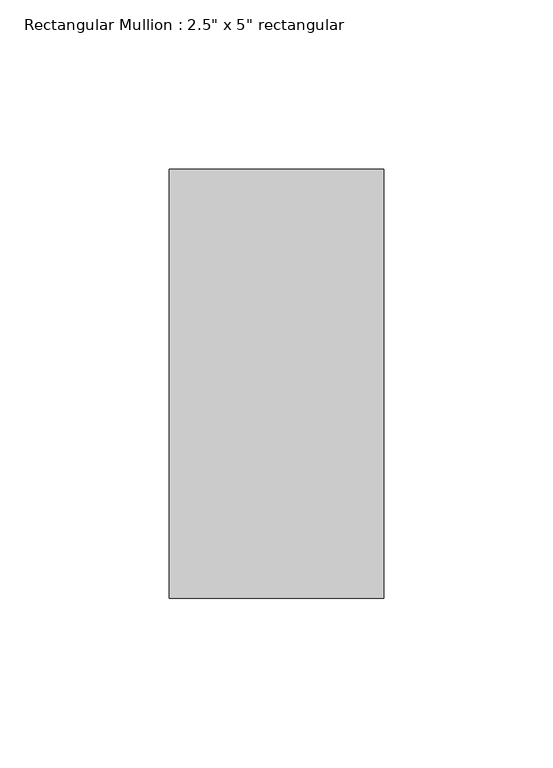
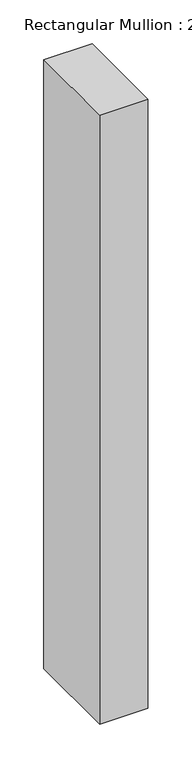
"""IFC4 building model written with IfcOpenShell, lengths in millimetres: member geometry."""

from ifc_helpers import new_model, si_unit, frame, origin, place, context, project, spatial, polyline, outline, extrude, source, transform, mapped, element, save


def member_8b2b7717(model_context):
    return source(origin(), model_context, "Body", "SweptSolid", [
        extrude(outline(polyline([(0.0, 63.5), (0.0, -63.5), (-63.5, -63.5), (-63.5, 63.5), (0.0, 63.5)])), frame((0.0, 0.0, -847.725), z_axis=(0.0, 0.0, 1.0), x_axis=(1.0, 0.0, 0.0)), (0.0, 0.0, 1.0), 847.725),
    ])


if __name__ == "__main__":
    model = new_model("IFC4")
    model_context = context("Model", 3, world=origin())
    ifc_project = project(units=[si_unit("LENGTHUNIT", "METRE", prefix="MILLI")], contexts=[model_context])
    site = spatial("IfcSite", under=ifc_project)
    building = spatial("IfcBuilding", under=site)
    placement = place(None, origin())
    member_shape = member_8b2b7717(model_context)
    element("IfcMember", 1, ObjectType="Rectangular Mullion : 2.5\" x 5\" rectangular", at=placement, inside=building, context=model_context, shape_type="MappedRepresentation", body=[
        mapped(member_shape, transform((0.0, 0.0, 0.0), x_axis=(1.0, 0.0, 0.0), y_axis=(0.0, 1.0, 0.0), z_axis=(0.0, 0.0, 1.0))),
    ])
    save(model, "model.ifc")

# Revit data of these elements
# Type "Rectangular Mullion : 2.5\" x 5\" rectangular"
#   built-in parameter 1007304 = 0.416667 (stored number, unit not read)
#   built-in parameter 1007301 = 0.104167 (stored number, unit not read)
#   built-in parameter 1007300 = 0.104167 (stored number, unit not read)
# Element 1 (IfcMember, "Rectangular Mullion : 2.5\" x 5\" rectangular")
#   Materials on its faces: "Aluminum"
# Materials
#   "Aluminum": class "Metal", colour RGB 247 247 247, transparency 0, Description = "Aluminum 6061", Cost = 0
